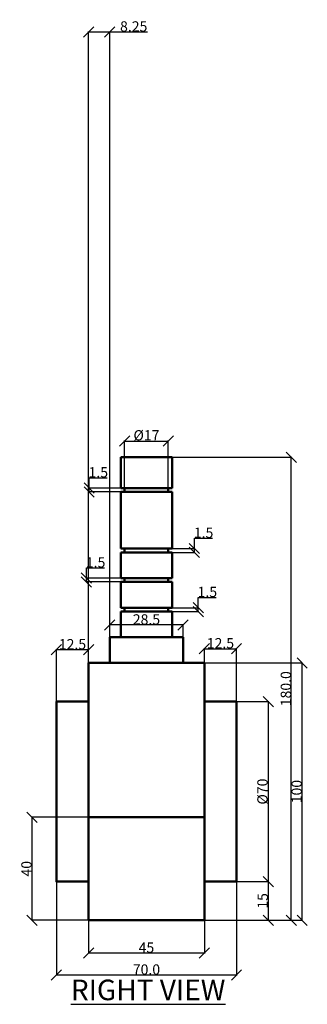
# Model space of a CAD drawing. Units: millimetres. Extents: x 2623 to 3019, y 2308 to 2699.
# Tile 3 of 3: x 2907 to 3019, y 2317 to 2699. Entities that reach past the tile are written whole.
import ezdxf

# ---------------------------------------------------------------- set-up
doc = ezdxf.new("R2010")
doc.units = ezdxf.units.MM
doc.header["$MEASUREMENT"] = 0
for name, color, linetype, lineweight in [('M-DIMS', 2, 'Continuous', 25), ('M-OUTL', 7, 'Continuous', 50), ('M-TEXT', 7, 'Continuous', 25)]:
    doc.layers.add(name, color=color, linetype=linetype, lineweight=lineweight)
doc.styles.get("Standard").update_dxf_attribs({"font": 'arial.ttf'})
doc.dimstyles.get("Standard").update_dxf_attribs({"dimtxt": 4, "dimasz": 4, "dimexe": 0.18, "dimexo": 0.0625, "dimgap": 0.09, "dimtad": 1, "dimtoh": 1, "dimdec": 0, "dimzin": 0, "dimdsep": 46, "dimtxsty": 'Standard', "dimblk": 'OBLIQUE', "dimcen": 0.09, "dimclre": 251, "dimadec": 0, "dimazin": 0, "dimtfac": 1, "dimtdec": 0, "dimtofl": 0, "dimtmove": 0, "dimatfit": 3, "dimfxl": 1, "dimtolj": 1, "dimtzin": 0, "dimarcsym": 0})

# ---------------------------------------------------------------- blocks, each defined once
blk = doc.blocks.new('_Oblique')
at = {"color": 0, "linetype": 'ByBlock', "lineweight": -2}
blk.add_line((-0.5, -0.5), (0.5, 0.5), dxfattribs=at)
blk = doc.blocks.new('*D20')
at = {"layer": 'Defpoints', "color": 0, "transparency": 16777216}
for p in [(2964.85, 2535.57), (2947.85, 2517.31), (2964.85, 2517.31)]:
    blk.add_point(p, dxfattribs=at)
at = {"layer": 'M-DIMS', "color": 0, "lineweight": -2, "transparency": 16777216}
for p, q in [((2947.85, 2517.37), (2947.85, 2535.75)), ((2947.85, 2535.57), (2964.85, 2535.57)), ((2964.85, 2517.37), (2964.85, 2535.75))]:
    blk.add_line(p, q, dxfattribs=at)
at = {"layer": 'M-DIMS', "color": 0, "lineweight": -2, "transparency": 16777216, "xscale": 4, "yscale": 4, "zscale": 4, "rotation": 180}
blk.add_blockref('_Oblique', (2947.85, 2535.57), dxfattribs=at)
at = {"layer": 'M-DIMS', "color": 0, "lineweight": -2, "transparency": 16777216, "xscale": 4, "yscale": 4, "zscale": 4}
blk.add_blockref('_Oblique', (2964.85, 2535.57), dxfattribs=at)
at = {"layer": 'M-DIMS', "color": 0, "transparency": 16777216, "insert": (2956.35, 2537.82), "char_height": 4, "attachment_point": 5}
blk.add_mtext('\\A1;%%C17', dxfattribs=at)
blk = doc.blocks.new('*D21')
at = {"layer": 'Defpoints', "color": 0, "transparency": 16777216}
for p in [(2934.08, 2517.31), (2946.35, 2517.31), (2946.35, 2515.81)]:
    blk.add_point(p, dxfattribs=at)
at = {"layer": 'M-DIMS', "color": 0, "lineweight": -2, "transparency": 16777216}
for p, q in [((2934.08, 2517.31), (2934.08, 2521.31)), ((2934.08, 2521.31), (2941.1, 2521.31)), ((2946.29, 2517.31), (2933.9, 2517.31)), ((2946.29, 2515.81), (2933.9, 2515.81)), ((2934.08, 2515.81), (2934.08, 2517.31))]:
    blk.add_line(p, q, dxfattribs=at)
at = {"layer": 'M-DIMS', "color": 0, "lineweight": -2, "transparency": 16777216, "xscale": 4, "yscale": 4, "zscale": 4}
for p, rotation in [((2934.08, 2517.31), 90), ((2934.08, 2515.81), 270)]:
    blk.add_blockref('_Oblique', p, dxfattribs=dict(at, rotation=rotation))
at = {"layer": 'M-DIMS', "color": 0, "transparency": 16777216, "insert": (2937.64, 2523.44), "char_height": 4, "attachment_point": 5}
blk.add_mtext('\\A1;1.5', dxfattribs=at)
blk = doc.blocks.new('*D22')
at = {"layer": 'Defpoints', "color": 0, "transparency": 16777216}
for p in [(2966.35, 2493.81), (2966.35, 2492.31), (2975.01, 2492.31)]:
    blk.add_point(p, dxfattribs=at)
at = {"layer": 'M-DIMS', "color": 0, "lineweight": -2, "transparency": 16777216}
for p, q in [((2975.01, 2493.81), (2975.01, 2497.81)), ((2975.01, 2497.81), (2982.03, 2497.81)), ((2966.41, 2493.81), (2975.19, 2493.81)), ((2966.41, 2492.31), (2975.19, 2492.31)), ((2975.01, 2492.31), (2975.01, 2493.81))]:
    blk.add_line(p, q, dxfattribs=at)
at = {"layer": 'M-DIMS', "color": 0, "lineweight": -2, "transparency": 16777216, "xscale": 4, "yscale": 4, "zscale": 4}
for p, rotation in [((2975.01, 2493.81), 90), ((2975.01, 2492.31), 270)]:
    blk.add_blockref('_Oblique', p, dxfattribs=dict(at, rotation=rotation))
at = {"layer": 'M-DIMS', "color": 0, "transparency": 16777216, "insert": (2978.56, 2499.94), "char_height": 4, "attachment_point": 5}
blk.add_mtext('\\A1;1.5', dxfattribs=at)
blk = doc.blocks.new('*D23')
at = {"layer": 'Defpoints', "color": 0, "transparency": 16777216}
for p in [(2933.03, 2482.31), (2946.35, 2482.31), (2946.35, 2480.81)]:
    blk.add_point(p, dxfattribs=at)
at = {"layer": 'M-DIMS', "color": 0, "lineweight": -2, "transparency": 16777216}
for p, q in [((2933.03, 2482.31), (2933.03, 2486.31)), ((2933.03, 2486.31), (2940.06, 2486.31)), ((2946.29, 2482.31), (2932.85, 2482.31)), ((2946.29, 2480.81), (2932.85, 2480.81)), ((2933.03, 2480.81), (2933.03, 2482.31))]:
    blk.add_line(p, q, dxfattribs=at)
at = {"layer": 'M-DIMS', "color": 0, "lineweight": -2, "transparency": 16777216, "xscale": 4, "yscale": 4, "zscale": 4}
for p, rotation in [((2933.03, 2482.31), 90), ((2933.03, 2480.81), 270)]:
    blk.add_blockref('_Oblique', p, dxfattribs=dict(at, rotation=rotation))
at = {"layer": 'M-DIMS', "color": 0, "transparency": 16777216, "insert": (2936.59, 2488.44), "char_height": 4, "attachment_point": 5}
blk.add_mtext('\\A1;1.5', dxfattribs=at)
blk = doc.blocks.new('*D24')
at = {"layer": 'Defpoints', "color": 0, "transparency": 16777216}
for p in [(2966.35, 2470.81), (2966.35, 2469.31), (2976.46, 2470.81)]:
    blk.add_point(p, dxfattribs=at)
at = {"layer": 'M-DIMS', "color": 0, "lineweight": -2, "transparency": 16777216}
for p, q in [((2976.46, 2470.81), (2976.46, 2474.81)), ((2976.46, 2474.81), (2983.49, 2474.81)), ((2966.41, 2470.81), (2976.64, 2470.81)), ((2966.41, 2469.31), (2976.64, 2469.31)), ((2976.46, 2469.31), (2976.46, 2470.81))]:
    blk.add_line(p, q, dxfattribs=at)
at = {"layer": 'M-DIMS', "color": 0, "lineweight": -2, "transparency": 16777216, "xscale": 4, "yscale": 4, "zscale": 4}
for p, rotation in [((2976.46, 2470.81), 90), ((2976.46, 2469.31), 270)]:
    blk.add_blockref('_Oblique', p, dxfattribs=dict(at, rotation=rotation))
at = {"layer": 'M-DIMS', "color": 0, "transparency": 16777216, "insert": (2980.02, 2476.94), "char_height": 4, "attachment_point": 5}
blk.add_mtext('\\A1;1.5', dxfattribs=at)
blk = doc.blocks.new('*D25')
at = {"layer": 'Defpoints', "color": 0, "transparency": 16777216}
for p in [(2942.1, 2464.11), (2942.1, 2459.31), (2970.6, 2459.31)]:
    blk.add_point(p, dxfattribs=at)
at = {"layer": 'M-DIMS', "color": 0, "lineweight": -2, "transparency": 16777216}
for p, q in [((2942.1, 2459.37), (2942.1, 2464.29)), ((2970.6, 2464.11), (2942.1, 2464.11)), ((2970.6, 2459.37), (2970.6, 2464.29))]:
    blk.add_line(p, q, dxfattribs=at)
at = {"layer": 'M-DIMS', "color": 0, "lineweight": -2, "transparency": 16777216, "xscale": 4, "yscale": 4, "zscale": 4, "rotation": 180}
blk.add_blockref('_Oblique', (2942.1, 2464.11), dxfattribs=at)
at = {"layer": 'M-DIMS', "color": 0, "lineweight": -2, "transparency": 16777216, "xscale": 4, "yscale": 4, "zscale": 4}
blk.add_blockref('_Oblique', (2970.6, 2464.11), dxfattribs=at)
at = {"layer": 'M-DIMS', "color": 0, "transparency": 16777216, "insert": (2956.35, 2466.24), "char_height": 4, "attachment_point": 5}
blk.add_mtext('\\A1;28.5', dxfattribs=at)
blk = doc.blocks.new('*D26')
at = {"layer": 'Defpoints', "color": 0, "transparency": 16777216}
for p in [(2921.35, 2454.47), (2933.85, 2449.31), (2921.35, 2434.31)]:
    blk.add_point(p, dxfattribs=at)
at = {"layer": 'M-DIMS', "color": 0, "lineweight": -2, "transparency": 16777216}
for p, q in [((2921.35, 2434.37), (2921.35, 2454.65)), ((2933.85, 2454.47), (2921.35, 2454.47)), ((2933.85, 2449.37), (2933.85, 2454.65))]:
    blk.add_line(p, q, dxfattribs=at)
at = {"layer": 'M-DIMS', "color": 0, "lineweight": -2, "transparency": 16777216, "xscale": 4, "yscale": 4, "zscale": 4, "rotation": 180}
blk.add_blockref('_Oblique', (2921.35, 2454.47), dxfattribs=at)
at = {"layer": 'M-DIMS', "color": 0, "lineweight": -2, "transparency": 16777216, "xscale": 4, "yscale": 4, "zscale": 4}
blk.add_blockref('_Oblique', (2933.85, 2454.47), dxfattribs=at)
at = {"layer": 'M-DIMS', "color": 0, "transparency": 16777216, "insert": (2927.6, 2456.61), "char_height": 4, "attachment_point": 5}
blk.add_mtext('\\A1;12.5', dxfattribs=at)
blk = doc.blocks.new('*D27')
at = {"layer": 'Defpoints', "color": 0, "transparency": 16777216}
for p in [(2991.35, 2454.85), (2978.85, 2449.31), (2991.35, 2434.31)]:
    blk.add_point(p, dxfattribs=at)
at = {"layer": 'M-DIMS', "color": 0, "lineweight": -2, "transparency": 16777216}
for p, q in [((2978.85, 2449.37), (2978.85, 2455.03)), ((2978.85, 2454.85), (2991.35, 2454.85)), ((2991.35, 2434.37), (2991.35, 2455.03))]:
    blk.add_line(p, q, dxfattribs=at)
at = {"layer": 'M-DIMS', "color": 0, "lineweight": -2, "transparency": 16777216, "xscale": 4, "yscale": 4, "zscale": 4, "rotation": 180}
blk.add_blockref('_Oblique', (2978.85, 2454.85), dxfattribs=at)
at = {"layer": 'M-DIMS', "color": 0, "lineweight": -2, "transparency": 16777216, "xscale": 4, "yscale": 4, "zscale": 4}
blk.add_blockref('_Oblique', (2991.35, 2454.85), dxfattribs=at)
at = {"layer": 'M-DIMS', "color": 0, "transparency": 16777216, "insert": (2985.1, 2456.99), "char_height": 4, "attachment_point": 5}
blk.add_mtext('\\A1;12.5', dxfattribs=at)
blk = doc.blocks.new('*D28')
at = {"layer": 'Defpoints', "color": 0, "transparency": 16777216}
for p in [(2991.35, 2434.31), (2991.35, 2364.31), (3003.67, 2364.31)]:
    blk.add_point(p, dxfattribs=at)
at = {"layer": 'M-DIMS', "color": 0, "lineweight": -2, "transparency": 16777216}
for p, q in [((2991.41, 2434.31), (3003.85, 2434.31)), ((3003.67, 2434.31), (3003.67, 2364.31)), ((2991.41, 2364.31), (3003.85, 2364.31))]:
    blk.add_line(p, q, dxfattribs=at)
at = {"layer": 'M-DIMS', "color": 0, "lineweight": -2, "transparency": 16777216, "xscale": 4, "yscale": 4, "zscale": 4}
for p, rotation in [((3003.67, 2434.31), 90), ((3003.67, 2364.31), 270)]:
    blk.add_blockref('_Oblique', p, dxfattribs=dict(at, rotation=rotation))
at = {"layer": 'M-DIMS', "color": 0, "transparency": 16777216, "insert": (3001.43, 2399.31), "char_height": 4, "attachment_point": 5, "rotation": 90}
blk.add_mtext('\\A1;%%C70', dxfattribs=at)
blk = doc.blocks.new('*D29')
at = {"layer": 'Defpoints', "color": 0, "transparency": 16777216}
for p in [(2978.85, 2449.31), (3016.86, 2449.31), (2978.85, 2349.31)]:
    blk.add_point(p, dxfattribs=at)
at = {"layer": 'M-DIMS', "color": 0, "lineweight": -2, "transparency": 16777216}
for p, q in [((2978.91, 2449.31), (3017.04, 2449.31)), ((3016.86, 2349.31), (3016.86, 2449.31)), ((2978.91, 2349.31), (3017.04, 2349.31))]:
    blk.add_line(p, q, dxfattribs=at)
at = {"layer": 'M-DIMS', "color": 0, "lineweight": -2, "transparency": 16777216, "xscale": 4, "yscale": 4, "zscale": 4}
for p, rotation in [((3016.86, 2449.31), 90), ((3016.86, 2349.31), 270)]:
    blk.add_blockref('_Oblique', p, dxfattribs=dict(at, rotation=rotation))
at = {"layer": 'M-DIMS', "color": 0, "transparency": 16777216, "insert": (3014.72, 2399.31), "char_height": 4, "attachment_point": 5, "rotation": 90}
blk.add_mtext('\\A1;100', dxfattribs=at)
blk = doc.blocks.new('*D30')
at = {"layer": 'Defpoints', "color": 0, "transparency": 16777216}
for p in [(2991.35, 2364.31), (2978.85, 2349.31), (3003.67, 2349.31)]:
    blk.add_point(p, dxfattribs=at)
at = {"layer": 'M-DIMS', "color": 0, "lineweight": -2, "transparency": 16777216}
for p, q in [((2991.41, 2364.31), (3003.85, 2364.31)), ((3003.67, 2364.31), (3003.67, 2349.31)), ((2978.91, 2349.31), (3003.85, 2349.31))]:
    blk.add_line(p, q, dxfattribs=at)
at = {"layer": 'M-DIMS', "color": 0, "lineweight": -2, "transparency": 16777216, "xscale": 4, "yscale": 4, "zscale": 4}
for p, rotation in [((3003.67, 2364.31), 90), ((3003.67, 2349.31), 270)]:
    blk.add_blockref('_Oblique', p, dxfattribs=dict(at, rotation=rotation))
at = {"layer": 'M-DIMS', "color": 0, "transparency": 16777216, "insert": (3001.54, 2356.81), "char_height": 4, "attachment_point": 5, "rotation": 90}
blk.add_mtext('\\A1;15', dxfattribs=at)
blk = doc.blocks.new('*D31')
at = {"layer": 'Defpoints', "color": 0, "transparency": 16777216}
for p in [(2933.85, 2349.31), (2978.85, 2349.31), (2933.85, 2336.53)]:
    blk.add_point(p, dxfattribs=at)
at = {"layer": 'M-DIMS', "color": 0, "lineweight": -2, "transparency": 16777216}
for p, q in [((2933.85, 2349.25), (2933.85, 2336.35)), ((2978.85, 2349.25), (2978.85, 2336.35)), ((2978.85, 2336.53), (2933.85, 2336.53))]:
    blk.add_line(p, q, dxfattribs=at)
at = {"layer": 'M-DIMS', "color": 0, "lineweight": -2, "transparency": 16777216, "xscale": 4, "yscale": 4, "zscale": 4, "rotation": 180}
blk.add_blockref('_Oblique', (2933.85, 2336.53), dxfattribs=at)
at = {"layer": 'M-DIMS', "color": 0, "lineweight": -2, "transparency": 16777216, "xscale": 4, "yscale": 4, "zscale": 4}
blk.add_blockref('_Oblique', (2978.85, 2336.53), dxfattribs=at)
at = {"layer": 'M-DIMS', "color": 0, "transparency": 16777216, "insert": (2956.35, 2338.65), "char_height": 4, "attachment_point": 5}
blk.add_mtext('\\A1;45', dxfattribs=at)
blk = doc.blocks.new('*D32')
at = {"layer": 'Defpoints', "color": 0, "transparency": 16777216}
for p in [(2933.85, 2389.31), (2911.85, 2349.31), (2933.85, 2349.31)]:
    blk.add_point(p, dxfattribs=at)
at = {"layer": 'M-DIMS', "color": 0, "lineweight": -2, "transparency": 16777216}
for p, q in [((2933.79, 2389.31), (2911.67, 2389.31)), ((2911.85, 2389.31), (2911.85, 2349.31)), ((2933.79, 2349.31), (2911.67, 2349.31))]:
    blk.add_line(p, q, dxfattribs=at)
at = {"layer": 'M-DIMS', "color": 0, "lineweight": -2, "transparency": 16777216, "xscale": 4, "yscale": 4, "zscale": 4}
for p, rotation in [((2911.85, 2389.31), 90), ((2911.85, 2349.31), 270)]:
    blk.add_blockref('_Oblique', p, dxfattribs=dict(at, rotation=rotation))
at = {"layer": 'M-DIMS', "color": 0, "transparency": 16777216, "insert": (2909.72, 2369.31), "char_height": 4, "attachment_point": 5, "rotation": 90}
blk.add_mtext('\\A1;40', dxfattribs=at)
blk = doc.blocks.new('SHAFT-GROOVED-END-ELEV')
for p, q in [((0, 60), (20, 60)), ((0, 48), (0, 60)), ((20, 48), (20, 60)), ((0, 48), (20, 48)), ((0, 46.5), (20, 46.5)), ((0, 24.5), (0, 46.5)), ((1.5, 46.5), (1.5, 48)), ((18.5, 46.5), (18.5, 48)), ((20, 24.5), (20, 46.5)), ((0, 24.5), (20, 24.5)), ((0, 23), (20, 23)), ((0, 13), (0, 23)), ((1.5, 23), (1.5, 24.5)), ((18.5, 23), (18.5, 24.5)), ((20, 13), (20, 23)), ((0, 13), (20, 13)), ((0, 11.5), (20, 11.5)), ((0, 1.5), (0, 11.5)), ((1.5, 11.5), (1.5, 13)), ((18.5, 11.5), (18.5, 13)), ((20, 1.5), (20, 11.5)), ((0, 1.5), (20, 1.5)), ((1.5, 0), (1.5, 1.5)), ((18.5, 1.5), (18.5, 0)), ((0, 0), (20, 0))]:
    blk.add_line(p, q)
blk = doc.blocks.new('*D48')
at = {"layer": 'Defpoints', "color": 0, "transparency": 16777216}
for p in [(2966.35, 2529.31), (3012.65, 2529.31), (2978.85, 2349.31)]:
    blk.add_point(p, dxfattribs=at)
at = {"layer": 'M-DIMS', "color": 251, "lineweight": -2, "transparency": 16777216}
for p, q in [((2966.41, 2529.31), (3012.83, 2529.31)), ((2978.91, 2349.31), (3012.83, 2349.31))]:
    blk.add_line(p, q, dxfattribs=at)
at = {"layer": 'M-DIMS', "color": 0, "lineweight": -2, "transparency": 16777216}
blk.add_line((3012.65, 2349.31), (3012.65, 2529.31), dxfattribs=at)
at = {"layer": 'M-DIMS', "color": 0, "lineweight": -2, "transparency": 16777216, "xscale": 4, "yscale": 4, "zscale": 4}
for p, rotation in [((3012.65, 2529.31), 90), ((3012.65, 2349.31), 270)]:
    blk.add_blockref('_Oblique', p, dxfattribs=dict(at, rotation=rotation))
at = {"layer": 'M-DIMS', "color": 0, "transparency": 16777216, "insert": (3010.52, 2439.31), "char_height": 4, "attachment_point": 5, "rotation": 90}
blk.add_mtext('\\A1;180.0', dxfattribs=at)
blk = doc.blocks.new('*D50')
at = {"layer": 'Defpoints', "color": 0, "transparency": 16777216}
for p in [(2942.1, 2694.64), (2942.1, 2459.31), (2933.85, 2449.31)]:
    blk.add_point(p, dxfattribs=at)
at = {"layer": 'M-DIMS', "color": 251, "lineweight": -2, "transparency": 16777216}
for p, q in [((2933.85, 2449.37), (2933.85, 2694.82)), ((2942.1, 2459.37), (2942.1, 2694.82))]:
    blk.add_line(p, q, dxfattribs=at)
at = {"layer": 'M-DIMS', "color": 0, "lineweight": -2, "transparency": 16777216}
for p, q in [((2933.85, 2694.64), (2942.1, 2694.64)), ((2942.1, 2694.64), (2956.71, 2694.64))]:
    blk.add_line(p, q, dxfattribs=at)
at = {"layer": 'M-DIMS', "color": 0, "lineweight": -2, "transparency": 16777216, "xscale": 4, "yscale": 4, "zscale": 4, "rotation": 180}
blk.add_blockref('_Oblique', (2933.85, 2694.64), dxfattribs=at)
at = {"layer": 'M-DIMS', "color": 0, "lineweight": -2, "transparency": 16777216, "xscale": 4, "yscale": 4, "zscale": 4}
blk.add_blockref('_Oblique', (2942.1, 2694.64), dxfattribs=at)
at = {"layer": 'M-DIMS', "color": 0, "transparency": 16777216, "insert": (2951.4, 2696.78), "char_height": 4, "attachment_point": 5}
blk.add_mtext('\\A1;8.25', dxfattribs=at)
blk = doc.blocks.new('*D51')
at = {"layer": 'Defpoints', "color": 0, "transparency": 16777216}
for p in [(2921.35, 2364.31), (2991.35, 2364.31), (2991.35, 2328.01)]:
    blk.add_point(p, dxfattribs=at)
at = {"layer": 'M-DIMS', "color": 251, "lineweight": -2, "transparency": 16777216}
for p, q in [((2921.35, 2364.25), (2921.35, 2327.83)), ((2991.35, 2364.25), (2991.35, 2327.83))]:
    blk.add_line(p, q, dxfattribs=at)
at = {"layer": 'M-DIMS', "color": 0, "lineweight": -2, "transparency": 16777216}
blk.add_line((2921.35, 2328.01), (2991.35, 2328.01), dxfattribs=at)
at = {"layer": 'M-DIMS', "color": 0, "lineweight": -2, "transparency": 16777216, "xscale": 4, "yscale": 4, "zscale": 4, "rotation": 180}
blk.add_blockref('_Oblique', (2921.35, 2328.01), dxfattribs=at)
at = {"layer": 'M-DIMS', "color": 0, "lineweight": -2, "transparency": 16777216, "xscale": 4, "yscale": 4, "zscale": 4}
blk.add_blockref('_Oblique', (2991.35, 2328.01), dxfattribs=at)
at = {"layer": 'M-DIMS', "color": 0, "transparency": 16777216, "insert": (2956.35, 2330.14), "char_height": 4, "attachment_point": 5}
blk.add_mtext('\\A1;70.0', dxfattribs=at)

msp = doc.modelspace()

# ---------------------------------------------------------------- linework, layer by layer
at = {"layer": 'M-OUTL'}
for p, q in [((2946.35, 2459.311), (2946.35, 2469.311)), ((2966.35, 2459.311), (2966.35, 2469.311)), ((2933.85, 2389.311), (2978.85, 2389.311))]:
    msp.add_line(p, q, dxfattribs=at)
for points in [[(2942.1, 2459.311), (2970.6, 2459.311), (2970.6, 2449.311), (2942.1, 2449.311)], [(2933.85, 2449.311), (2978.85, 2449.311), (2978.85, 2349.311), (2933.85, 2349.311)], [(2921.35, 2434.311), (2933.85, 2434.311), (2933.85, 2364.311), (2921.35, 2364.311)], [(2978.85, 2434.311), (2991.35, 2434.311), (2991.35, 2364.311), (2978.85, 2364.311)]]:
    msp.add_lwpolyline(points, close=True, dxfattribs=at)

# ---------------------------------------------------------------- block references
msp.add_blockref('SHAFT-GROOVED-END-ELEV', (2946.35, 2469.311), dxfattribs=at)

# ---------------------------------------------------------------- texts
at = {"layer": 'M-TEXT', "insert": (2926.962, 2326.209), "char_height": 8, "attachment_point": 1}
msp.add_mtext_dynamic_manual_height_columns('{\\LRIGHT VIEW}', width=72.37298, gutter_width=1, heights=[0], dxfattribs=at)

# ---------------------------------------------------------------- dimensions: what is measured, and where the dimension line sits
at = {"layer": 'M-DIMS'}
for base, p1, p2, override, picture, middle in [((2942.1, 2694.644), (2933.85, 2449.311), (2942.1, 2459.311), {"dimdec": 2, "dimlfac": 1, "dimrnd": 0, "dimzin": 0, "dimdsep": 46, "dimlunit": 2}, '*D50', (2951.403, 2696.776)), ((2942.1, 2464.112), (2970.6, 2459.311), (2942.1, 2459.311), {"dimdec": 1, "dimclrd": 0, "dimclre": 0, "dimclrt": 0}, '*D25', (2956.35, 2466.245)), ((2921.35, 2454.474), (2933.85, 2449.311), (2921.35, 2434.311), {"dimdec": 1, "dimclrd": 0, "dimclre": 0, "dimclrt": 0}, '*D26', (2927.6, 2456.606)), ((2991.35, 2454.854), (2978.85, 2449.311), (2991.35, 2434.311), {"dimdec": 1, "dimclrd": 0, "dimclre": 0, "dimclrt": 0}, '*D27', (2985.1, 2456.986)), ((2991.35, 2328.011), (2921.35, 2364.311), (2991.35, 2364.311), {"dimdec": 1, "dimlfac": 1, "dimrnd": 0, "dimzin": 0, "dimdsep": 46, "dimlunit": 2}, '*D51', (2956.35, 2330.143)), ((2933.85, 2336.53), (2978.85, 2349.311), (2933.85, 2349.311), {"dimclrd": 0, "dimclre": 0, "dimclrt": 0}, '*D31', (2956.35, 2338.654))]:
    dim = msp.add_linear_dim(base=base, p1=p1, p2=p2, dimstyle='Standard', override=override, dxfattribs=at)
    dim.commit()
    dim.dimension.update_dxf_attribs({"geometry": picture, "text_midpoint": middle})
dim = msp.add_linear_dim(base=(2964.85, 2535.574), p1=(2947.85, 2517.311), p2=(2964.85, 2517.311), text='%%C<>', dimstyle='Standard', override={"dimclrd": 0, "dimclre": 0, "dimclrt": 0}, dxfattribs=at)
dim.commit()
dim.dimension.update_dxf_attribs({"geometry": '*D20', "text_midpoint": (2956.35, 2537.818)})
for base, p1, p2, override, picture, middle in [((3012.65, 2529.311), (2978.85, 2349.311), (2966.35, 2529.311), {"dimdec": 1, "dimlfac": 1, "dimrnd": 0, "dimzin": 0, "dimdsep": 46, "dimlunit": 2}, '*D48', (3010.518, 2439.311)), ((2934.078, 2517.311), (2946.35, 2515.811), (2946.35, 2517.311), {"dimdec": 1, "dimclrd": 0, "dimclre": 0, "dimclrt": 0}, '*D21', (2937.636, 2523.443)), ((2933.032, 2482.311), (2946.35, 2480.811), (2946.35, 2482.311), {"dimdec": 1, "dimclrd": 0, "dimclre": 0, "dimclrt": 0}, '*D23', (2936.59, 2488.443)), ((2976.462, 2470.811), (2966.35, 2469.311), (2966.35, 2470.811), {"dimdec": 1, "dimclrd": 0, "dimclre": 0, "dimclrt": 0}, '*D24', (2980.02, 2476.943)), ((3016.856, 2449.311), (2978.85, 2349.311), (2978.85, 2449.311), {"dimclrd": 0, "dimclre": 0, "dimclrt": 0}, '*D29', (3014.723, 2399.311)), ((2911.849, 2349.311), (2933.85, 2389.311), (2933.85, 2349.311), {"dimclrd": 0, "dimclre": 0, "dimclrt": 0}, '*D32', (2909.717, 2369.311)), ((3003.675, 2349.311), (2991.35, 2364.311), (2978.85, 2349.311), {"dimclrd": 0, "dimclre": 0, "dimclrt": 0}, '*D30', (3001.543, 2356.811))]:
    dim = msp.add_linear_dim(base=base, p1=p1, p2=p2, angle=90, dimstyle='Standard', override=override, dxfattribs=at)
    dim.commit()
    dim.dimension.update_dxf_attribs({"geometry": picture, "text_midpoint": middle})
dim = msp.add_linear_dim(base=(2975.006, 2492.311), p1=(2966.35, 2493.811), p2=(2966.35, 2492.311), angle=90, dimstyle='Standard', override={"dimdec": 1, "dimclrd": 0, "dimclre": 0, "dimclrt": 0}, dxfattribs=at)
dim.commit()
dim.dimension.update_dxf_attribs({"geometry": '*D22', "text_midpoint": (2978.564, 2497.811), "dimtype": 160})
dim = msp.add_linear_dim(base=(3003.675, 2364.311), p1=(2991.35, 2434.311), p2=(2991.35, 2364.311), angle=90, text='%%C<>', dimstyle='Standard', override={"dimclrd": 0, "dimclre": 0, "dimclrt": 0}, dxfattribs=at)
dim.commit()
dim.dimension.update_dxf_attribs({"geometry": '*D28', "text_midpoint": (3001.431, 2399.311)})

doc.saveas('drawing.dxf')
